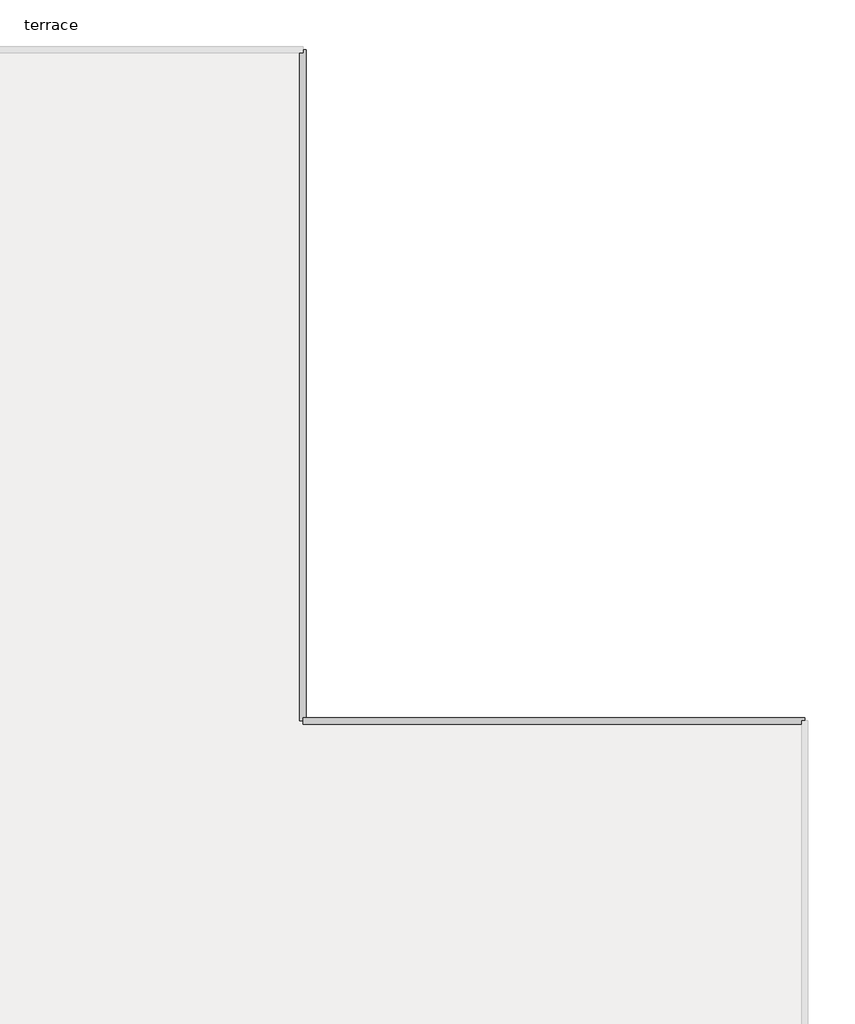
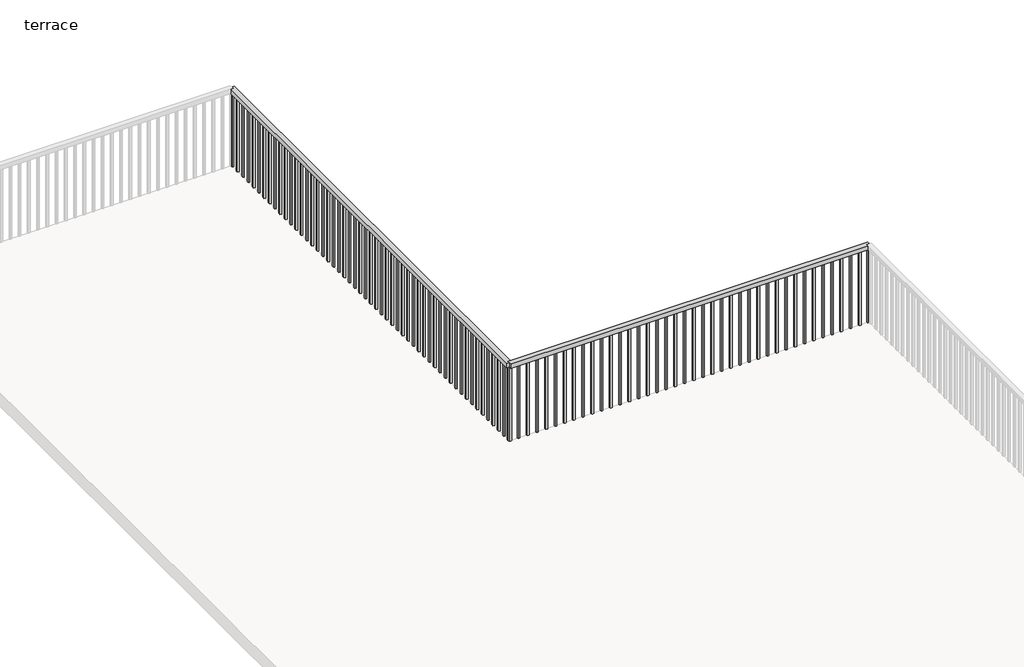
# One storey, part 4 of 4: 2 railings.
"""IFC4 building model written with IfcOpenShell, lengths in millimetres."""

from ifc_helpers import new_model, si_unit, frame, origin, place, context, project, spatial, polyline, outline, extrude, element, save

model = new_model("IFC4")

# Units and contexts
model_context = context("Model", 3, world=origin())
ifc_project = project(units=[si_unit("LENGTHUNIT", "METRE", prefix="MILLI")], contexts=[model_context])

# Site, building, storey
site = spatial("IfcSite", under=ifc_project)
building = spatial("IfcBuilding", under=site)
storey = spatial("IfcBuildingStorey", under=building, Name="terrace", Elevation=7010.4)

# Railings
placement = place(None, origin())
element("IfcRailing", 1, ObjectType="Handrail - Rectangular", at=placement, inside=storey, context=model_context, shape_type="SweptSolid", body=[
    extrude(outline(polyline([(32217.7316163, 14362.3980552), (32166.9316163, 14362.3980552), (32166.9316163, 19658.2980552), (32217.7316163, 19658.2980552), (32217.7316163, 14362.3980552)])), frame((0.0, 0.0, 7874.0), z_axis=(0.0, 0.0, 1.0), x_axis=(1.0, 0.0, 0.0)), (0.0, 0.0, 1.0), 50.8),
    extrude(outline(polyline([(32201.8566163, 19636.0730552), (32182.8066163, 19636.0730552), (32182.8066163, 19655.1230552), (32201.8566163, 19655.1230552), (32201.8566163, 19636.0730552)])), frame((0.0, 0.0, 7010.4), z_axis=(0.0, 0.0, 1.0), x_axis=(1.0, 0.0, 0.0)), (0.0, 0.0, 1.0), 863.6),
    extrude(outline(polyline([(32201.8566163, 19534.4730552), (32182.8066163, 19534.4730552), (32182.8066163, 19553.5230552), (32201.8566163, 19553.5230552), (32201.8566163, 19534.4730552)])), frame((0.0, 0.0, 7010.4), z_axis=(0.0, 0.0, 1.0), x_axis=(1.0, 0.0, 0.0)), (0.0, 0.0, 1.0), 863.6),
    extrude(outline(polyline([(32201.8566163, 19432.8730552), (32182.8066163, 19432.8730552), (32182.8066163, 19451.9230552), (32201.8566163, 19451.9230552), (32201.8566163, 19432.8730552)])), frame((0.0, 0.0, 7010.4), z_axis=(0.0, 0.0, 1.0), x_axis=(1.0, 0.0, 0.0)), (0.0, 0.0, 1.0), 863.6),
    extrude(outline(polyline([(32201.8566163, 19331.2730552), (32182.8066163, 19331.2730552), (32182.8066163, 19350.3230552), (32201.8566163, 19350.3230552), (32201.8566163, 19331.2730552)])), frame((0.0, 0.0, 7010.4), z_axis=(0.0, 0.0, 1.0), x_axis=(1.0, 0.0, 0.0)), (0.0, 0.0, 1.0), 863.6),
    extrude(outline(polyline([(32201.8566163, 19229.6730552), (32182.8066163, 19229.6730552), (32182.8066163, 19248.7230552), (32201.8566163, 19248.7230552), (32201.8566163, 19229.6730552)])), frame((0.0, 0.0, 7010.4), z_axis=(0.0, 0.0, 1.0), x_axis=(1.0, 0.0, 0.0)), (0.0, 0.0, 1.0), 863.6),
    extrude(outline(polyline([(32201.8566163, 19128.0730552), (32182.8066163, 19128.0730552), (32182.8066163, 19147.1230552), (32201.8566163, 19147.1230552), (32201.8566163, 19128.0730552)])), frame((0.0, 0.0, 7010.4), z_axis=(0.0, 0.0, 1.0), x_axis=(1.0, 0.0, 0.0)), (0.0, 0.0, 1.0), 863.6),
    extrude(outline(polyline([(32201.8566163, 19026.4730552), (32182.8066163, 19026.4730552), (32182.8066163, 19045.5230552), (32201.8566163, 19045.5230552), (32201.8566163, 19026.4730552)])), frame((0.0, 0.0, 7010.4), z_axis=(0.0, 0.0, 1.0), x_axis=(1.0, 0.0, 0.0)), (0.0, 0.0, 1.0), 863.6),
    extrude(outline(polyline([(32201.8566163, 18924.8730552), (32182.8066163, 18924.8730552), (32182.8066163, 18943.9230552), (32201.8566163, 18943.9230552), (32201.8566163, 18924.8730552)])), frame((0.0, 0.0, 7010.4), z_axis=(0.0, 0.0, 1.0), x_axis=(1.0, 0.0, 0.0)), (0.0, 0.0, 1.0), 863.6),
    extrude(outline(polyline([(32201.8566163, 18823.2730552), (32182.8066163, 18823.2730552), (32182.8066163, 18842.3230552), (32201.8566163, 18842.3230552), (32201.8566163, 18823.2730552)])), frame((0.0, 0.0, 7010.4), z_axis=(0.0, 0.0, 1.0), x_axis=(1.0, 0.0, 0.0)), (0.0, 0.0, 1.0), 863.6),
    extrude(outline(polyline([(32201.8566163, 18721.6730552), (32182.8066163, 18721.6730552), (32182.8066163, 18740.7230552), (32201.8566163, 18740.7230552), (32201.8566163, 18721.6730552)])), frame((0.0, 0.0, 7010.4), z_axis=(0.0, 0.0, 1.0), x_axis=(1.0, 0.0, 0.0)), (0.0, 0.0, 1.0), 863.6),
    extrude(outline(polyline([(32201.8566163, 18620.0730552), (32182.8066163, 18620.0730552), (32182.8066163, 18639.1230552), (32201.8566163, 18639.1230552), (32201.8566163, 18620.0730552)])), frame((0.0, 0.0, 7010.4), z_axis=(0.0, 0.0, 1.0), x_axis=(1.0, 0.0, 0.0)), (0.0, 0.0, 1.0), 863.6),
    extrude(outline(polyline([(32201.8566163, 18518.4730552), (32182.8066163, 18518.4730552), (32182.8066163, 18537.5230552), (32201.8566163, 18537.5230552), (32201.8566163, 18518.4730552)])), frame((0.0, 0.0, 7010.4), z_axis=(0.0, 0.0, 1.0), x_axis=(1.0, 0.0, 0.0)), (0.0, 0.0, 1.0), 863.6),
    extrude(outline(polyline([(32201.8566163, 18416.8730552), (32182.8066163, 18416.8730552), (32182.8066163, 18435.9230552), (32201.8566163, 18435.9230552), (32201.8566163, 18416.8730552)])), frame((0.0, 0.0, 7010.4), z_axis=(0.0, 0.0, 1.0), x_axis=(1.0, 0.0, 0.0)), (0.0, 0.0, 1.0), 863.6),
    extrude(outline(polyline([(32201.8566163, 18315.2730552), (32182.8066163, 18315.2730552), (32182.8066163, 18334.3230552), (32201.8566163, 18334.3230552), (32201.8566163, 18315.2730552)])), frame((0.0, 0.0, 7010.4), z_axis=(0.0, 0.0, 1.0), x_axis=(1.0, 0.0, 0.0)), (0.0, 0.0, 1.0), 863.6),
    extrude(outline(polyline([(32201.8566163, 18213.6730552), (32182.8066163, 18213.6730552), (32182.8066163, 18232.7230552), (32201.8566163, 18232.7230552), (32201.8566163, 18213.6730552)])), frame((0.0, 0.0, 7010.4), z_axis=(0.0, 0.0, 1.0), x_axis=(1.0, 0.0, 0.0)), (0.0, 0.0, 1.0), 863.6),
    extrude(outline(polyline([(32201.8566163, 18112.0730552), (32182.8066163, 18112.0730552), (32182.8066163, 18131.1230552), (32201.8566163, 18131.1230552), (32201.8566163, 18112.0730552)])), frame((0.0, 0.0, 7010.4), z_axis=(0.0, 0.0, 1.0), x_axis=(1.0, 0.0, 0.0)), (0.0, 0.0, 1.0), 863.6),
    extrude(outline(polyline([(32201.8566163, 18010.4730552), (32182.8066163, 18010.4730552), (32182.8066163, 18029.5230552), (32201.8566163, 18029.5230552), (32201.8566163, 18010.4730552)])), frame((0.0, 0.0, 7010.4), z_axis=(0.0, 0.0, 1.0), x_axis=(1.0, 0.0, 0.0)), (0.0, 0.0, 1.0), 863.6),
    extrude(outline(polyline([(32201.8566163, 17908.8730552), (32182.8066163, 17908.8730552), (32182.8066163, 17927.9230552), (32201.8566163, 17927.9230552), (32201.8566163, 17908.8730552)])), frame((0.0, 0.0, 7010.4), z_axis=(0.0, 0.0, 1.0), x_axis=(1.0, 0.0, 0.0)), (0.0, 0.0, 1.0), 863.6),
    extrude(outline(polyline([(32201.8566163, 17807.2730552), (32182.8066163, 17807.2730552), (32182.8066163, 17826.3230552), (32201.8566163, 17826.3230552), (32201.8566163, 17807.2730552)])), frame((0.0, 0.0, 7010.4), z_axis=(0.0, 0.0, 1.0), x_axis=(1.0, 0.0, 0.0)), (0.0, 0.0, 1.0), 863.6),
    extrude(outline(polyline([(32201.8566163, 17705.6730552), (32182.8066163, 17705.6730552), (32182.8066163, 17724.7230552), (32201.8566163, 17724.7230552), (32201.8566163, 17705.6730552)])), frame((0.0, 0.0, 7010.4), z_axis=(0.0, 0.0, 1.0), x_axis=(1.0, 0.0, 0.0)), (0.0, 0.0, 1.0), 863.6),
    extrude(outline(polyline([(32201.8566163, 17604.0730552), (32182.8066163, 17604.0730552), (32182.8066163, 17623.1230552), (32201.8566163, 17623.1230552), (32201.8566163, 17604.0730552)])), frame((0.0, 0.0, 7010.4), z_axis=(0.0, 0.0, 1.0), x_axis=(1.0, 0.0, 0.0)), (0.0, 0.0, 1.0), 863.6),
    extrude(outline(polyline([(32201.8566163, 17502.4730552), (32182.8066163, 17502.4730552), (32182.8066163, 17521.5230552), (32201.8566163, 17521.5230552), (32201.8566163, 17502.4730552)])), frame((0.0, 0.0, 7010.4), z_axis=(0.0, 0.0, 1.0), x_axis=(1.0, 0.0, 0.0)), (0.0, 0.0, 1.0), 863.6),
    extrude(outline(polyline([(32201.8566163, 17400.8730552), (32182.8066163, 17400.8730552), (32182.8066163, 17419.9230552), (32201.8566163, 17419.9230552), (32201.8566163, 17400.8730552)])), frame((0.0, 0.0, 7010.4), z_axis=(0.0, 0.0, 1.0), x_axis=(1.0, 0.0, 0.0)), (0.0, 0.0, 1.0), 863.6),
    extrude(outline(polyline([(32201.8566163, 17299.2730552), (32182.8066163, 17299.2730552), (32182.8066163, 17318.3230552), (32201.8566163, 17318.3230552), (32201.8566163, 17299.2730552)])), frame((0.0, 0.0, 7010.4), z_axis=(0.0, 0.0, 1.0), x_axis=(1.0, 0.0, 0.0)), (0.0, 0.0, 1.0), 863.6),
    extrude(outline(polyline([(32201.8566163, 17197.6730552), (32182.8066163, 17197.6730552), (32182.8066163, 17216.7230552), (32201.8566163, 17216.7230552), (32201.8566163, 17197.6730552)])), frame((0.0, 0.0, 7010.4), z_axis=(0.0, 0.0, 1.0), x_axis=(1.0, 0.0, 0.0)), (0.0, 0.0, 1.0), 863.6),
    extrude(outline(polyline([(32201.8566163, 17096.0730552), (32182.8066163, 17096.0730552), (32182.8066163, 17115.1230552), (32201.8566163, 17115.1230552), (32201.8566163, 17096.0730552)])), frame((0.0, 0.0, 7010.4), z_axis=(0.0, 0.0, 1.0), x_axis=(1.0, 0.0, 0.0)), (0.0, 0.0, 1.0), 863.6),
    extrude(outline(polyline([(32201.8566163, 16994.4730552), (32182.8066163, 16994.4730552), (32182.8066163, 17013.5230552), (32201.8566163, 17013.5230552), (32201.8566163, 16994.4730552)])), frame((0.0, 0.0, 7010.4), z_axis=(0.0, 0.0, 1.0), x_axis=(1.0, 0.0, 0.0)), (0.0, 0.0, 1.0), 863.6),
    extrude(outline(polyline([(32201.8566163, 16892.8730552), (32182.8066163, 16892.8730552), (32182.8066163, 16911.9230552), (32201.8566163, 16911.9230552), (32201.8566163, 16892.8730552)])), frame((0.0, 0.0, 7010.4), z_axis=(0.0, 0.0, 1.0), x_axis=(1.0, 0.0, 0.0)), (0.0, 0.0, 1.0), 863.6),
    extrude(outline(polyline([(32201.8566163, 16791.2730552), (32182.8066163, 16791.2730552), (32182.8066163, 16810.3230552), (32201.8566163, 16810.3230552), (32201.8566163, 16791.2730552)])), frame((0.0, 0.0, 7010.4), z_axis=(0.0, 0.0, 1.0), x_axis=(1.0, 0.0, 0.0)), (0.0, 0.0, 1.0), 863.6),
    extrude(outline(polyline([(32201.8566163, 16689.6730552), (32182.8066163, 16689.6730552), (32182.8066163, 16708.7230552), (32201.8566163, 16708.7230552), (32201.8566163, 16689.6730552)])), frame((0.0, 0.0, 7010.4), z_axis=(0.0, 0.0, 1.0), x_axis=(1.0, 0.0, 0.0)), (0.0, 0.0, 1.0), 863.6),
    extrude(outline(polyline([(32201.8566163, 16588.0730552), (32182.8066163, 16588.0730552), (32182.8066163, 16607.1230552), (32201.8566163, 16607.1230552), (32201.8566163, 16588.0730552)])), frame((0.0, 0.0, 7010.4), z_axis=(0.0, 0.0, 1.0), x_axis=(1.0, 0.0, 0.0)), (0.0, 0.0, 1.0), 863.6),
    extrude(outline(polyline([(32201.8566163, 16486.4730552), (32182.8066163, 16486.4730552), (32182.8066163, 16505.5230552), (32201.8566163, 16505.5230552), (32201.8566163, 16486.4730552)])), frame((0.0, 0.0, 7010.4), z_axis=(0.0, 0.0, 1.0), x_axis=(1.0, 0.0, 0.0)), (0.0, 0.0, 1.0), 863.6),
    extrude(outline(polyline([(32201.8566163, 16384.8730552), (32182.8066163, 16384.8730552), (32182.8066163, 16403.9230552), (32201.8566163, 16403.9230552), (32201.8566163, 16384.8730552)])), frame((0.0, 0.0, 7010.4), z_axis=(0.0, 0.0, 1.0), x_axis=(1.0, 0.0, 0.0)), (0.0, 0.0, 1.0), 863.6),
    extrude(outline(polyline([(32201.8566163, 16283.2730552), (32182.8066163, 16283.2730552), (32182.8066163, 16302.3230552), (32201.8566163, 16302.3230552), (32201.8566163, 16283.2730552)])), frame((0.0, 0.0, 7010.4), z_axis=(0.0, 0.0, 1.0), x_axis=(1.0, 0.0, 0.0)), (0.0, 0.0, 1.0), 863.6),
    extrude(outline(polyline([(32201.8566163, 16181.6730552), (32182.8066163, 16181.6730552), (32182.8066163, 16200.7230552), (32201.8566163, 16200.7230552), (32201.8566163, 16181.6730552)])), frame((0.0, 0.0, 7010.4), z_axis=(0.0, 0.0, 1.0), x_axis=(1.0, 0.0, 0.0)), (0.0, 0.0, 1.0), 863.6),
    extrude(outline(polyline([(32201.8566163, 16080.0730552), (32182.8066163, 16080.0730552), (32182.8066163, 16099.1230552), (32201.8566163, 16099.1230552), (32201.8566163, 16080.0730552)])), frame((0.0, 0.0, 7010.4), z_axis=(0.0, 0.0, 1.0), x_axis=(1.0, 0.0, 0.0)), (0.0, 0.0, 1.0), 863.6),
    extrude(outline(polyline([(32201.8566163, 15978.4730552), (32182.8066163, 15978.4730552), (32182.8066163, 15997.5230552), (32201.8566163, 15997.5230552), (32201.8566163, 15978.4730552)])), frame((0.0, 0.0, 7010.4), z_axis=(0.0, 0.0, 1.0), x_axis=(1.0, 0.0, 0.0)), (0.0, 0.0, 1.0), 863.6),
    extrude(outline(polyline([(32201.8566163, 15876.8730552), (32182.8066163, 15876.8730552), (32182.8066163, 15895.9230552), (32201.8566163, 15895.9230552), (32201.8566163, 15876.8730552)])), frame((0.0, 0.0, 7010.4), z_axis=(0.0, 0.0, 1.0), x_axis=(1.0, 0.0, 0.0)), (0.0, 0.0, 1.0), 863.6),
    extrude(outline(polyline([(32201.8566163, 15775.2730552), (32182.8066163, 15775.2730552), (32182.8066163, 15794.3230552), (32201.8566163, 15794.3230552), (32201.8566163, 15775.2730552)])), frame((0.0, 0.0, 7010.4), z_axis=(0.0, 0.0, 1.0), x_axis=(1.0, 0.0, 0.0)), (0.0, 0.0, 1.0), 863.6),
    extrude(outline(polyline([(32201.8566163, 15673.6730552), (32182.8066163, 15673.6730552), (32182.8066163, 15692.7230552), (32201.8566163, 15692.7230552), (32201.8566163, 15673.6730552)])), frame((0.0, 0.0, 7010.4), z_axis=(0.0, 0.0, 1.0), x_axis=(1.0, 0.0, 0.0)), (0.0, 0.0, 1.0), 863.6),
    extrude(outline(polyline([(32201.8566163, 15572.0730552), (32182.8066163, 15572.0730552), (32182.8066163, 15591.1230552), (32201.8566163, 15591.1230552), (32201.8566163, 15572.0730552)])), frame((0.0, 0.0, 7010.4), z_axis=(0.0, 0.0, 1.0), x_axis=(1.0, 0.0, 0.0)), (0.0, 0.0, 1.0), 863.6),
    extrude(outline(polyline([(32201.8566163, 15470.4730552), (32182.8066163, 15470.4730552), (32182.8066163, 15489.5230552), (32201.8566163, 15489.5230552), (32201.8566163, 15470.4730552)])), frame((0.0, 0.0, 7010.4), z_axis=(0.0, 0.0, 1.0), x_axis=(1.0, 0.0, 0.0)), (0.0, 0.0, 1.0), 863.6),
    extrude(outline(polyline([(32201.8566163, 15368.8730552), (32182.8066163, 15368.8730552), (32182.8066163, 15387.9230552), (32201.8566163, 15387.9230552), (32201.8566163, 15368.8730552)])), frame((0.0, 0.0, 7010.4), z_axis=(0.0, 0.0, 1.0), x_axis=(1.0, 0.0, 0.0)), (0.0, 0.0, 1.0), 863.6),
    extrude(outline(polyline([(32201.8566163, 15267.2730552), (32182.8066163, 15267.2730552), (32182.8066163, 15286.3230552), (32201.8566163, 15286.3230552), (32201.8566163, 15267.2730552)])), frame((0.0, 0.0, 7010.4), z_axis=(0.0, 0.0, 1.0), x_axis=(1.0, 0.0, 0.0)), (0.0, 0.0, 1.0), 863.6),
    extrude(outline(polyline([(32201.8566163, 15165.6730552), (32182.8066163, 15165.6730552), (32182.8066163, 15184.7230552), (32201.8566163, 15184.7230552), (32201.8566163, 15165.6730552)])), frame((0.0, 0.0, 7010.4), z_axis=(0.0, 0.0, 1.0), x_axis=(1.0, 0.0, 0.0)), (0.0, 0.0, 1.0), 863.6),
    extrude(outline(polyline([(32201.8566163, 15064.0730552), (32182.8066163, 15064.0730552), (32182.8066163, 15083.1230552), (32201.8566163, 15083.1230552), (32201.8566163, 15064.0730552)])), frame((0.0, 0.0, 7010.4), z_axis=(0.0, 0.0, 1.0), x_axis=(1.0, 0.0, 0.0)), (0.0, 0.0, 1.0), 863.6),
    extrude(outline(polyline([(32201.8566163, 14962.4730552), (32182.8066163, 14962.4730552), (32182.8066163, 14981.5230552), (32201.8566163, 14981.5230552), (32201.8566163, 14962.4730552)])), frame((0.0, 0.0, 7010.4), z_axis=(0.0, 0.0, 1.0), x_axis=(1.0, 0.0, 0.0)), (0.0, 0.0, 1.0), 863.6),
    extrude(outline(polyline([(32201.8566163, 14860.8730552), (32182.8066163, 14860.8730552), (32182.8066163, 14879.9230552), (32201.8566163, 14879.9230552), (32201.8566163, 14860.8730552)])), frame((0.0, 0.0, 7010.4), z_axis=(0.0, 0.0, 1.0), x_axis=(1.0, 0.0, 0.0)), (0.0, 0.0, 1.0), 863.6),
    extrude(outline(polyline([(32201.8566163, 14759.2730552), (32182.8066163, 14759.2730552), (32182.8066163, 14778.3230552), (32201.8566163, 14778.3230552), (32201.8566163, 14759.2730552)])), frame((0.0, 0.0, 7010.4), z_axis=(0.0, 0.0, 1.0), x_axis=(1.0, 0.0, 0.0)), (0.0, 0.0, 1.0), 863.6),
    extrude(outline(polyline([(32201.8566163, 14657.6730552), (32182.8066163, 14657.6730552), (32182.8066163, 14676.7230552), (32201.8566163, 14676.7230552), (32201.8566163, 14657.6730552)])), frame((0.0, 0.0, 7010.4), z_axis=(0.0, 0.0, 1.0), x_axis=(1.0, 0.0, 0.0)), (0.0, 0.0, 1.0), 863.6),
    extrude(outline(polyline([(32201.8566163, 14556.0730552), (32182.8066163, 14556.0730552), (32182.8066163, 14575.1230552), (32201.8566163, 14575.1230552), (32201.8566163, 14556.0730552)])), frame((0.0, 0.0, 7010.4), z_axis=(0.0, 0.0, 1.0), x_axis=(1.0, 0.0, 0.0)), (0.0, 0.0, 1.0), 863.6),
    extrude(outline(polyline([(32201.8566163, 14454.4730552), (32182.8066163, 14454.4730552), (32182.8066163, 14473.5230552), (32201.8566163, 14473.5230552), (32201.8566163, 14454.4730552)])), frame((0.0, 0.0, 7010.4), z_axis=(0.0, 0.0, 1.0), x_axis=(1.0, 0.0, 0.0)), (0.0, 0.0, 1.0), 863.6),
    extrude(outline(polyline([(32201.8566163, 19639.2480552), (32182.8066163, 19639.2480552), (32182.8066163, 19658.2980552), (32201.8566163, 19658.2980552), (32201.8566163, 19639.2480552)])), frame((0.0, 0.0, 7010.4), z_axis=(0.0, 0.0, 1.0), x_axis=(1.0, 0.0, 0.0)), (0.0, 0.0, 1.0), 863.6),
    extrude(outline(polyline([(32201.8566163, 14362.3980552), (32182.8066163, 14362.3980552), (32182.8066163, 14381.4480552), (32201.8566163, 14381.4480552), (32201.8566163, 14362.3980552)])), frame((0.0, 0.0, 7010.4), z_axis=(0.0, 0.0, 1.0), x_axis=(1.0, 0.0, 0.0)), (0.0, 0.0, 1.0), 863.6),
])
element("IfcRailing", 2, ObjectType="Handrail - Rectangular", at=placement, inside=storey, context=model_context, shape_type="SweptSolid", body=[
    extrude(outline(polyline([(36154.7316163, 14387.7980552), (36154.7316163, 14336.9980552), (32192.3316163, 14336.9980552), (32192.3316163, 14387.7980552), (36154.7316163, 14387.7980552)])), frame((0.0, 0.0, 7874.0), z_axis=(0.0, 0.0, 1.0), x_axis=(1.0, 0.0, 0.0)), (0.0, 0.0, 1.0), 50.8),
    extrude(outline(polyline([(32303.4566163, 14371.9230552), (32303.4566163, 14352.8730552), (32284.4066163, 14352.8730552), (32284.4066163, 14371.9230552), (32303.4566163, 14371.9230552)])), frame((0.0, 0.0, 7010.4), z_axis=(0.0, 0.0, 1.0), x_axis=(1.0, 0.0, 0.0)), (0.0, 0.0, 1.0), 863.6),
    extrude(outline(polyline([(32405.0566163, 14371.9230552), (32405.0566163, 14352.8730552), (32386.0066163, 14352.8730552), (32386.0066163, 14371.9230552), (32405.0566163, 14371.9230552)])), frame((0.0, 0.0, 7010.4), z_axis=(0.0, 0.0, 1.0), x_axis=(1.0, 0.0, 0.0)), (0.0, 0.0, 1.0), 863.6),
    extrude(outline(polyline([(32506.6566163, 14371.9230552), (32506.6566163, 14352.8730552), (32487.6066163, 14352.8730552), (32487.6066163, 14371.9230552), (32506.6566163, 14371.9230552)])), frame((0.0, 0.0, 7010.4), z_axis=(0.0, 0.0, 1.0), x_axis=(1.0, 0.0, 0.0)), (0.0, 0.0, 1.0), 863.6),
    extrude(outline(polyline([(32608.2566163, 14371.9230552), (32608.2566163, 14352.8730552), (32589.2066163, 14352.8730552), (32589.2066163, 14371.9230552), (32608.2566163, 14371.9230552)])), frame((0.0, 0.0, 7010.4), z_axis=(0.0, 0.0, 1.0), x_axis=(1.0, 0.0, 0.0)), (0.0, 0.0, 1.0), 863.6),
    extrude(outline(polyline([(32709.8566163, 14371.9230552), (32709.8566163, 14352.8730552), (32690.8066163, 14352.8730552), (32690.8066163, 14371.9230552), (32709.8566163, 14371.9230552)])), frame((0.0, 0.0, 7010.4), z_axis=(0.0, 0.0, 1.0), x_axis=(1.0, 0.0, 0.0)), (0.0, 0.0, 1.0), 863.6),
    extrude(outline(polyline([(32811.4566163, 14371.9230552), (32811.4566163, 14352.8730552), (32792.4066163, 14352.8730552), (32792.4066163, 14371.9230552), (32811.4566163, 14371.9230552)])), frame((0.0, 0.0, 7010.4), z_axis=(0.0, 0.0, 1.0), x_axis=(1.0, 0.0, 0.0)), (0.0, 0.0, 1.0), 863.6),
    extrude(outline(polyline([(32913.0566163, 14371.9230552), (32913.0566163, 14352.8730552), (32894.0066163, 14352.8730552), (32894.0066163, 14371.9230552), (32913.0566163, 14371.9230552)])), frame((0.0, 0.0, 7010.4), z_axis=(0.0, 0.0, 1.0), x_axis=(1.0, 0.0, 0.0)), (0.0, 0.0, 1.0), 863.6),
    extrude(outline(polyline([(33014.6566163, 14371.9230552), (33014.6566163, 14352.8730552), (32995.6066163, 14352.8730552), (32995.6066163, 14371.9230552), (33014.6566163, 14371.9230552)])), frame((0.0, 0.0, 7010.4), z_axis=(0.0, 0.0, 1.0), x_axis=(1.0, 0.0, 0.0)), (0.0, 0.0, 1.0), 863.6),
    extrude(outline(polyline([(33116.2566163, 14371.9230552), (33116.2566163, 14352.8730552), (33097.2066163, 14352.8730552), (33097.2066163, 14371.9230552), (33116.2566163, 14371.9230552)])), frame((0.0, 0.0, 7010.4), z_axis=(0.0, 0.0, 1.0), x_axis=(1.0, 0.0, 0.0)), (0.0, 0.0, 1.0), 863.6),
    extrude(outline(polyline([(33217.8566163, 14371.9230552), (33217.8566163, 14352.8730552), (33198.8066163, 14352.8730552), (33198.8066163, 14371.9230552), (33217.8566163, 14371.9230552)])), frame((0.0, 0.0, 7010.4), z_axis=(0.0, 0.0, 1.0), x_axis=(1.0, 0.0, 0.0)), (0.0, 0.0, 1.0), 863.6),
    extrude(outline(polyline([(33319.4566163, 14371.9230552), (33319.4566163, 14352.8730552), (33300.4066163, 14352.8730552), (33300.4066163, 14371.9230552), (33319.4566163, 14371.9230552)])), frame((0.0, 0.0, 7010.4), z_axis=(0.0, 0.0, 1.0), x_axis=(1.0, 0.0, 0.0)), (0.0, 0.0, 1.0), 863.6),
    extrude(outline(polyline([(33421.0566163, 14371.9230552), (33421.0566163, 14352.8730552), (33402.0066163, 14352.8730552), (33402.0066163, 14371.9230552), (33421.0566163, 14371.9230552)])), frame((0.0, 0.0, 7010.4), z_axis=(0.0, 0.0, 1.0), x_axis=(1.0, 0.0, 0.0)), (0.0, 0.0, 1.0), 863.6),
    extrude(outline(polyline([(33522.6566163, 14371.9230552), (33522.6566163, 14352.8730552), (33503.6066163, 14352.8730552), (33503.6066163, 14371.9230552), (33522.6566163, 14371.9230552)])), frame((0.0, 0.0, 7010.4), z_axis=(0.0, 0.0, 1.0), x_axis=(1.0, 0.0, 0.0)), (0.0, 0.0, 1.0), 863.6),
    extrude(outline(polyline([(33624.2566163, 14371.9230552), (33624.2566163, 14352.8730552), (33605.2066163, 14352.8730552), (33605.2066163, 14371.9230552), (33624.2566163, 14371.9230552)])), frame((0.0, 0.0, 7010.4), z_axis=(0.0, 0.0, 1.0), x_axis=(1.0, 0.0, 0.0)), (0.0, 0.0, 1.0), 863.6),
    extrude(outline(polyline([(33725.8566163, 14371.9230552), (33725.8566163, 14352.8730552), (33706.8066163, 14352.8730552), (33706.8066163, 14371.9230552), (33725.8566163, 14371.9230552)])), frame((0.0, 0.0, 7010.4), z_axis=(0.0, 0.0, 1.0), x_axis=(1.0, 0.0, 0.0)), (0.0, 0.0, 1.0), 863.6),
    extrude(outline(polyline([(33827.4566163, 14371.9230552), (33827.4566163, 14352.8730552), (33808.4066163, 14352.8730552), (33808.4066163, 14371.9230552), (33827.4566163, 14371.9230552)])), frame((0.0, 0.0, 7010.4), z_axis=(0.0, 0.0, 1.0), x_axis=(1.0, 0.0, 0.0)), (0.0, 0.0, 1.0), 863.6),
    extrude(outline(polyline([(33929.0566163, 14371.9230552), (33929.0566163, 14352.8730552), (33910.0066163, 14352.8730552), (33910.0066163, 14371.9230552), (33929.0566163, 14371.9230552)])), frame((0.0, 0.0, 7010.4), z_axis=(0.0, 0.0, 1.0), x_axis=(1.0, 0.0, 0.0)), (0.0, 0.0, 1.0), 863.6),
    extrude(outline(polyline([(34030.6566163, 14371.9230552), (34030.6566163, 14352.8730552), (34011.6066163, 14352.8730552), (34011.6066163, 14371.9230552), (34030.6566163, 14371.9230552)])), frame((0.0, 0.0, 7010.4), z_axis=(0.0, 0.0, 1.0), x_axis=(1.0, 0.0, 0.0)), (0.0, 0.0, 1.0), 863.6),
    extrude(outline(polyline([(34132.2566163, 14371.9230552), (34132.2566163, 14352.8730552), (34113.2066163, 14352.8730552), (34113.2066163, 14371.9230552), (34132.2566163, 14371.9230552)])), frame((0.0, 0.0, 7010.4), z_axis=(0.0, 0.0, 1.0), x_axis=(1.0, 0.0, 0.0)), (0.0, 0.0, 1.0), 863.6),
    extrude(outline(polyline([(34233.8566163, 14371.9230552), (34233.8566163, 14352.8730552), (34214.8066163, 14352.8730552), (34214.8066163, 14371.9230552), (34233.8566163, 14371.9230552)])), frame((0.0, 0.0, 7010.4), z_axis=(0.0, 0.0, 1.0), x_axis=(1.0, 0.0, 0.0)), (0.0, 0.0, 1.0), 863.6),
    extrude(outline(polyline([(34335.4566163, 14371.9230552), (34335.4566163, 14352.8730552), (34316.4066163, 14352.8730552), (34316.4066163, 14371.9230552), (34335.4566163, 14371.9230552)])), frame((0.0, 0.0, 7010.4), z_axis=(0.0, 0.0, 1.0), x_axis=(1.0, 0.0, 0.0)), (0.0, 0.0, 1.0), 863.6),
    extrude(outline(polyline([(34437.0566163, 14371.9230552), (34437.0566163, 14352.8730552), (34418.0066163, 14352.8730552), (34418.0066163, 14371.9230552), (34437.0566163, 14371.9230552)])), frame((0.0, 0.0, 7010.4), z_axis=(0.0, 0.0, 1.0), x_axis=(1.0, 0.0, 0.0)), (0.0, 0.0, 1.0), 863.6),
    extrude(outline(polyline([(34538.6566163, 14371.9230552), (34538.6566163, 14352.8730552), (34519.6066163, 14352.8730552), (34519.6066163, 14371.9230552), (34538.6566163, 14371.9230552)])), frame((0.0, 0.0, 7010.4), z_axis=(0.0, 0.0, 1.0), x_axis=(1.0, 0.0, 0.0)), (0.0, 0.0, 1.0), 863.6),
    extrude(outline(polyline([(34640.2566163, 14371.9230552), (34640.2566163, 14352.8730552), (34621.2066163, 14352.8730552), (34621.2066163, 14371.9230552), (34640.2566163, 14371.9230552)])), frame((0.0, 0.0, 7010.4), z_axis=(0.0, 0.0, 1.0), x_axis=(1.0, 0.0, 0.0)), (0.0, 0.0, 1.0), 863.6),
    extrude(outline(polyline([(34741.8566163, 14371.9230552), (34741.8566163, 14352.8730552), (34722.8066163, 14352.8730552), (34722.8066163, 14371.9230552), (34741.8566163, 14371.9230552)])), frame((0.0, 0.0, 7010.4), z_axis=(0.0, 0.0, 1.0), x_axis=(1.0, 0.0, 0.0)), (0.0, 0.0, 1.0), 863.6),
    extrude(outline(polyline([(34843.4566163, 14371.9230552), (34843.4566163, 14352.8730552), (34824.4066163, 14352.8730552), (34824.4066163, 14371.9230552), (34843.4566163, 14371.9230552)])), frame((0.0, 0.0, 7010.4), z_axis=(0.0, 0.0, 1.0), x_axis=(1.0, 0.0, 0.0)), (0.0, 0.0, 1.0), 863.6),
    extrude(outline(polyline([(34945.0566163, 14371.9230552), (34945.0566163, 14352.8730552), (34926.0066163, 14352.8730552), (34926.0066163, 14371.9230552), (34945.0566163, 14371.9230552)])), frame((0.0, 0.0, 7010.4), z_axis=(0.0, 0.0, 1.0), x_axis=(1.0, 0.0, 0.0)), (0.0, 0.0, 1.0), 863.6),
    extrude(outline(polyline([(35046.6566163, 14371.9230552), (35046.6566163, 14352.8730552), (35027.6066163, 14352.8730552), (35027.6066163, 14371.9230552), (35046.6566163, 14371.9230552)])), frame((0.0, 0.0, 7010.4), z_axis=(0.0, 0.0, 1.0), x_axis=(1.0, 0.0, 0.0)), (0.0, 0.0, 1.0), 863.6),
    extrude(outline(polyline([(35148.2566163, 14371.9230552), (35148.2566163, 14352.8730552), (35129.2066163, 14352.8730552), (35129.2066163, 14371.9230552), (35148.2566163, 14371.9230552)])), frame((0.0, 0.0, 7010.4), z_axis=(0.0, 0.0, 1.0), x_axis=(1.0, 0.0, 0.0)), (0.0, 0.0, 1.0), 863.6),
    extrude(outline(polyline([(35249.8566163, 14371.9230552), (35249.8566163, 14352.8730552), (35230.8066163, 14352.8730552), (35230.8066163, 14371.9230552), (35249.8566163, 14371.9230552)])), frame((0.0, 0.0, 7010.4), z_axis=(0.0, 0.0, 1.0), x_axis=(1.0, 0.0, 0.0)), (0.0, 0.0, 1.0), 863.6),
    extrude(outline(polyline([(35351.4566163, 14371.9230552), (35351.4566163, 14352.8730552), (35332.4066163, 14352.8730552), (35332.4066163, 14371.9230552), (35351.4566163, 14371.9230552)])), frame((0.0, 0.0, 7010.4), z_axis=(0.0, 0.0, 1.0), x_axis=(1.0, 0.0, 0.0)), (0.0, 0.0, 1.0), 863.6),
    extrude(outline(polyline([(35453.0566163, 14371.9230552), (35453.0566163, 14352.8730552), (35434.0066163, 14352.8730552), (35434.0066163, 14371.9230552), (35453.0566163, 14371.9230552)])), frame((0.0, 0.0, 7010.4), z_axis=(0.0, 0.0, 1.0), x_axis=(1.0, 0.0, 0.0)), (0.0, 0.0, 1.0), 863.6),
    extrude(outline(polyline([(35554.6566163, 14371.9230552), (35554.6566163, 14352.8730552), (35535.6066163, 14352.8730552), (35535.6066163, 14371.9230552), (35554.6566163, 14371.9230552)])), frame((0.0, 0.0, 7010.4), z_axis=(0.0, 0.0, 1.0), x_axis=(1.0, 0.0, 0.0)), (0.0, 0.0, 1.0), 863.6),
    extrude(outline(polyline([(35656.2566163, 14371.9230552), (35656.2566163, 14352.8730552), (35637.2066163, 14352.8730552), (35637.2066163, 14371.9230552), (35656.2566163, 14371.9230552)])), frame((0.0, 0.0, 7010.4), z_axis=(0.0, 0.0, 1.0), x_axis=(1.0, 0.0, 0.0)), (0.0, 0.0, 1.0), 863.6),
    extrude(outline(polyline([(35757.8566163, 14371.9230552), (35757.8566163, 14352.8730552), (35738.8066163, 14352.8730552), (35738.8066163, 14371.9230552), (35757.8566163, 14371.9230552)])), frame((0.0, 0.0, 7010.4), z_axis=(0.0, 0.0, 1.0), x_axis=(1.0, 0.0, 0.0)), (0.0, 0.0, 1.0), 863.6),
    extrude(outline(polyline([(35859.4566163, 14371.9230552), (35859.4566163, 14352.8730552), (35840.4066163, 14352.8730552), (35840.4066163, 14371.9230552), (35859.4566163, 14371.9230552)])), frame((0.0, 0.0, 7010.4), z_axis=(0.0, 0.0, 1.0), x_axis=(1.0, 0.0, 0.0)), (0.0, 0.0, 1.0), 863.6),
    extrude(outline(polyline([(35961.0566163, 14371.9230552), (35961.0566163, 14352.8730552), (35942.0066163, 14352.8730552), (35942.0066163, 14371.9230552), (35961.0566163, 14371.9230552)])), frame((0.0, 0.0, 7010.4), z_axis=(0.0, 0.0, 1.0), x_axis=(1.0, 0.0, 0.0)), (0.0, 0.0, 1.0), 863.6),
    extrude(outline(polyline([(36062.6566163, 14371.9230552), (36062.6566163, 14352.8730552), (36043.6066163, 14352.8730552), (36043.6066163, 14371.9230552), (36062.6566163, 14371.9230552)])), frame((0.0, 0.0, 7010.4), z_axis=(0.0, 0.0, 1.0), x_axis=(1.0, 0.0, 0.0)), (0.0, 0.0, 1.0), 863.6),
    extrude(outline(polyline([(32211.3816163, 14371.9230552), (32211.3816163, 14352.8730552), (32192.3316163, 14352.8730552), (32192.3316163, 14371.9230552), (32211.3816163, 14371.9230552)])), frame((0.0, 0.0, 7010.4), z_axis=(0.0, 0.0, 1.0), x_axis=(1.0, 0.0, 0.0)), (0.0, 0.0, 1.0), 863.6),
    extrude(outline(polyline([(36154.7316163, 14371.9230552), (36154.7316163, 14352.8730552), (36135.6816163, 14352.8730552), (36135.6816163, 14371.9230552), (36154.7316163, 14371.9230552)])), frame((0.0, 0.0, 7010.4), z_axis=(0.0, 0.0, 1.0), x_axis=(1.0, 0.0, 0.0)), (0.0, 0.0, 1.0), 863.6),
])

save(model, "model.ifc")

# Revit data of these elements
# Type "Handrail - Rectangular"
#   Assembly Code = "C2010400"
#   built-in parameter 1008612 = 0.0416667 (stored number, unit not read)
#   built-in parameter 1008611 = 0.0416667 (stored number, unit not read)
#   built-in parameter 1008609 = 0.333333 (stored number, unit not read)
#   built-in parameter 1008604 = 0.166667 (stored number, unit not read)
#   built-in parameter 1008603 = 0.166667 (stored number, unit not read)
#   Railing Height = 3' - 0"
#   built-in parameter 1008630 = 2
#   built-in parameter 1008610 = 2
#   built-in parameter 1008618 = Baluster - Square : 3/4"
# Elements 1, 2 (IfcRailing, "Handrail - Rectangular")
#   Phase Created = New Construction
